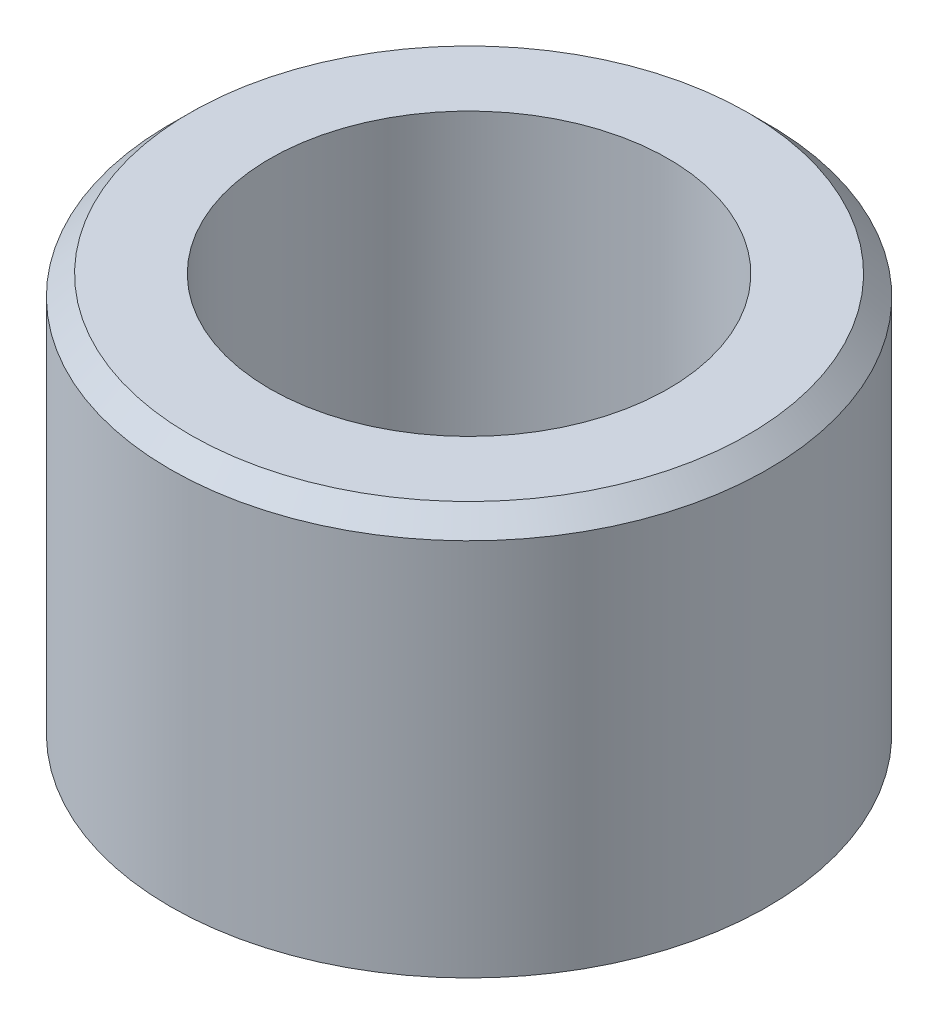
ISO-10303-21;
HEADER;
FILE_DESCRIPTION(('STEP AP214'),'2;1');
FILE_NAME('part.step','',(''),(''),'','','');
FILE_SCHEMA(('AUTOMOTIVE_DESIGN { 1 0 10303 214 1 1 1 1 }'));
ENDSEC;
DATA;
#1=APPLICATION_CONTEXT('core data for automotive mechanical design processes');
#2=APPLICATION_PROTOCOL_DEFINITION('international standard','automotive_design',2000,#1);
#3=PRODUCT_CONTEXT('',#1,'mechanical');
#4=PRODUCT('Part','Part','',(#3));
#5=PRODUCT_RELATED_PRODUCT_CATEGORY('part','',(#4));
#6=PRODUCT_DEFINITION_FORMATION('','',#4);
#7=PRODUCT_DEFINITION_CONTEXT('part definition',#1,'design');
#8=PRODUCT_DEFINITION('design','',#6,#7);
#9=PRODUCT_DEFINITION_SHAPE('','',#8);
#10=(LENGTH_UNIT() NAMED_UNIT(*) SI_UNIT(.MILLI.,.METRE.));
#11=(NAMED_UNIT(*) PLANE_ANGLE_UNIT() SI_UNIT($,.RADIAN.));
#12=(NAMED_UNIT(*) SI_UNIT($,.STERADIAN.) SOLID_ANGLE_UNIT());
#13=UNCERTAINTY_MEASURE_WITH_UNIT(LENGTH_MEASURE(1.E-05),#10,'distance_accuracy_value','');
#14=(GEOMETRIC_REPRESENTATION_CONTEXT(3) GLOBAL_UNCERTAINTY_ASSIGNED_CONTEXT((#13)) GLOBAL_UNIT_ASSIGNED_CONTEXT((#10,
#11,#12)) REPRESENTATION_CONTEXT('',''));
#15=CARTESIAN_POINT('',(0.,0.,0.));
#16=DIRECTION('',(0.,0.,1.));
#17=DIRECTION('',(1.,0.,0.));
#18=AXIS2_PLACEMENT_3D('',#15,#16,#17);
#19=CARTESIAN_POINT('',(0.,20.,0.));
#20=DIRECTION('',(0.,1.,0.));
#21=DIRECTION('',(0.,0.,1.));
#22=AXIS2_PLACEMENT_3D('',#19,#20,#21);
#23=PLANE('',#22);
#24=CARTESIAN_POINT('',(0.,20.,0.));
#25=DIRECTION('',(0.,1.,0.));
#26=DIRECTION('',(0.,0.,1.));
#27=AXIS2_PLACEMENT_3D('',#24,#25,#26);
#28=CIRCLE('',#27,14.);
#29=CARTESIAN_POINT('',(0.,20.,14.));
#30=VERTEX_POINT('',#29);
#31=EDGE_CURVE('E51',#30,#30,#28,.T.);
#32=ORIENTED_EDGE('',*,*,#31,.T.);
#33=EDGE_LOOP('',(#32));
#34=FACE_BOUND('',#33,.T.);
#35=CARTESIAN_POINT('',(0.,20.,0.));
#36=DIRECTION('',(0.,1.,0.));
#37=DIRECTION('',(0.,0.,1.));
#38=AXIS2_PLACEMENT_3D('',#35,#36,#37);
#39=CIRCLE('',#38,10.);
#40=CARTESIAN_POINT('',(0.,20.,10.));
#41=VERTEX_POINT('',#40);
#42=EDGE_CURVE('E56',#41,#41,#39,.T.);
#43=ORIENTED_EDGE('',*,*,#42,.F.);
#44=EDGE_LOOP('',(#43));
#45=FACE_BOUND('',#44,.T.);
#46=ADVANCED_FACE('F43',(#34,#45),#23,.T.);
#47=CARTESIAN_POINT('',(0.,0.,0.));
#48=DIRECTION('',(0.,1.,0.));
#49=DIRECTION('',(0.,0.,1.));
#50=AXIS2_PLACEMENT_3D('',#47,#48,#49);
#51=PLANE('',#50);
#52=CARTESIAN_POINT('',(0.,0.,0.));
#53=DIRECTION('',(0.,1.,0.));
#54=DIRECTION('',(0.,0.,1.));
#55=AXIS2_PLACEMENT_3D('',#52,#53,#54);
#56=CIRCLE('',#55,15.);
#57=CARTESIAN_POINT('',(0.,0.,15.));
#58=VERTEX_POINT('',#57);
#59=EDGE_CURVE('E54',#58,#58,#56,.T.);
#60=ORIENTED_EDGE('',*,*,#59,.F.);
#61=EDGE_LOOP('',(#60));
#62=FACE_BOUND('',#61,.T.);
#63=CARTESIAN_POINT('',(0.,0.,0.));
#64=DIRECTION('',(0.,1.,0.));
#65=DIRECTION('',(0.,0.,1.));
#66=AXIS2_PLACEMENT_3D('',#63,#64,#65);
#67=CIRCLE('',#66,10.);
#68=CARTESIAN_POINT('',(0.,0.,10.));
#69=VERTEX_POINT('',#68);
#70=EDGE_CURVE('E61',#69,#69,#67,.T.);
#71=ORIENTED_EDGE('',*,*,#70,.T.);
#72=EDGE_LOOP('',(#71));
#73=FACE_BOUND('',#72,.T.);
#74=ADVANCED_FACE('F75',(#62,#73),#51,.F.);
#75=CARTESIAN_POINT('',(0.,20.,0.));
#76=DIRECTION('',(0.,-1.,0.));
#77=DIRECTION('',(0.,0.,-1.));
#78=AXIS2_PLACEMENT_3D('',#75,#76,#77);
#79=CYLINDRICAL_SURFACE('',#78,15.);
#80=CARTESIAN_POINT('',(0.,19.,0.));
#81=DIRECTION('',(0.,1.,0.));
#82=DIRECTION('',(0.,0.,1.));
#83=AXIS2_PLACEMENT_3D('',#80,#81,#82);
#84=CIRCLE('',#83,15.);
#85=CARTESIAN_POINT('',(0.,19.,15.));
#86=VERTEX_POINT('',#85);
#87=EDGE_CURVE('E10',#86,#86,#84,.F.);
#88=ORIENTED_EDGE('',*,*,#87,.T.);
#89=EDGE_LOOP('',(#88));
#90=FACE_BOUND('',#89,.T.);
#91=ORIENTED_EDGE('',*,*,#59,.T.);
#92=EDGE_LOOP('',(#91));
#93=FACE_BOUND('',#92,.T.);
#94=ADVANCED_FACE('F76',(#90,#93),#79,.T.);
#95=CARTESIAN_POINT('',(0.,20.,0.));
#96=DIRECTION('',(0.,-1.,0.));
#97=DIRECTION('',(0.,0.,-1.));
#98=AXIS2_PLACEMENT_3D('',#95,#96,#97);
#99=CYLINDRICAL_SURFACE('',#98,10.);
#100=ORIENTED_EDGE('',*,*,#42,.T.);
#101=EDGE_LOOP('',(#100));
#102=FACE_BOUND('',#101,.T.);
#103=ORIENTED_EDGE('',*,*,#70,.F.);
#104=EDGE_LOOP('',(#103));
#105=FACE_BOUND('',#104,.T.);
#106=ADVANCED_FACE('F66',(#102,#105),#99,.F.);
#107=CARTESIAN_POINT('',(0.,20.,0.));
#108=DIRECTION('',(0.,-1.,0.));
#109=DIRECTION('',(0.,0.,-1.));
#110=AXIS2_PLACEMENT_3D('',#107,#108,#109);
#111=CONICAL_SURFACE('',#110,14.,0.785398163397446);
#112=ORIENTED_EDGE('',*,*,#87,.F.);
#113=EDGE_LOOP('',(#112));
#114=FACE_BOUND('',#113,.T.);
#115=ORIENTED_EDGE('',*,*,#31,.F.);
#116=EDGE_LOOP('',(#115));
#117=FACE_BOUND('',#116,.T.);
#118=ADVANCED_FACE('F46',(#114,#117),#111,.T.);
#119=CLOSED_SHELL('',(#46,#74,#94,#106,#118));
#120=MANIFOLD_SOLID_BREP('B2',#119);
#121=ADVANCED_BREP_SHAPE_REPRESENTATION('',(#18,#120),#14);
#122=SHAPE_DEFINITION_REPRESENTATION(#9,#121);
ENDSEC;
END-ISO-10303-21;
